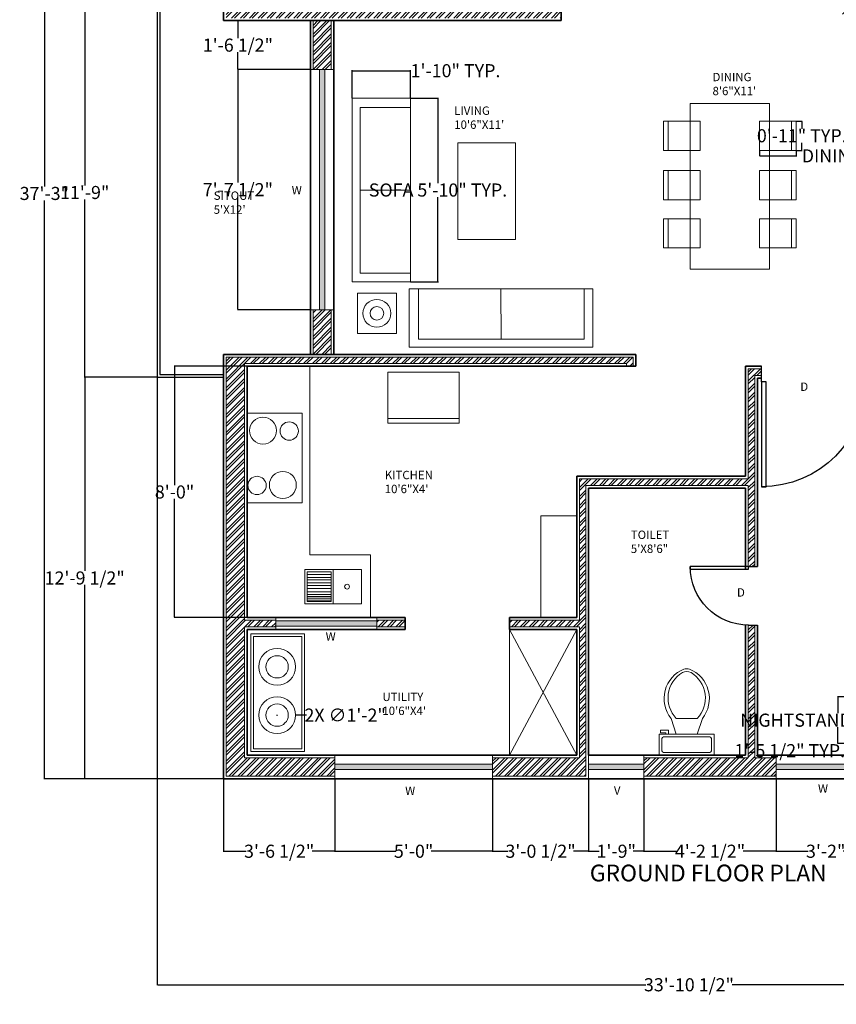
# Model space of a CAD drawing. Units: inches. Extents: x -340 to 394, y 381 to 1380.
# Tile 1 of 3: x -117 to 195, y 381 to 757. Entities that reach past the tile are written whole.
import ezdxf

# ---------------------------------------------------------------- set-up
doc = ezdxf.new("R2010")
doc.units = ezdxf.units.IN
doc.header["$MEASUREMENT"] = 0
for name, color, linetype, lineweight in [('A-ANNO-DIMS', 150, 'Continuous', 18), ('A-ANNO-TEXT', 11, 'Continuous', 18), ('A-AREA-IDEN', 11, 'Continuous', 18), ('A-EQPM', 130, 'Continuous', 18), ('A-FLOR', 150, 'Continuous', 25), ('A-FLOR-CASE', 130, 'Continuous', 20), ('A-FLOR-FIXT', 130, 'Continuous', 18), ('A-GLAZ-PATT', 220, 'Continuous', 13), ('A-WALL-FNSH', 150, 'Continuous', 18), ('A-WALL-PATT', 10, 'Continuous', 13), ('door', 200, 'Continuous', 25), ('fur', 130, 'Continuous', 18), ('wall', 150, 'Continuous', 35), ('wind', 220, 'Continuous', 20)]:
    doc.layers.add(name, color=color, linetype=linetype, lineweight=lineweight)
doc.styles.get("Standard").update_dxf_attribs({"font": 'arial.ttf'})
doc.dimstyles.get("Standard").update_dxf_attribs({"dimtxt": 5, "dimasz": 0.18, "dimexe": 0.18, "dimexo": 0.0625, "dimgap": 0.09, "dimtad": 0, "dimtih": 1, "dimtoh": 1, "dimdec": 0, "dimzin": 0, "dimdsep": 46, "dimlunit": 4, "dimtxsty": 'Standard', "dimcen": 0.09, "dimadec": 0, "dimazin": 0, "dimtfac": 1, "dimtdec": 0, "dimtofl": 0, "dimtmove": 0, "dimatfit": 3, "dimfxl": 1, "dimtolj": 1, "dimtzin": 0, "dimarcsym": 0})

# ---------------------------------------------------------------- blocks, each defined once
blk = doc.blocks.new('*U2')
for p, q in [((0, 0), (0, -6)), ((40, 0), (40, -6))]:
    blk.add_line(p, q)
blk.add_lwpolyline([(0, 0), (0, 40), (1.75, 40), (1.75, 0)], close=True)
blk.add_arc((0, 0), 40, 0, 90)
blk = doc.blocks.new('*U4')
for p, q in [((9.5, -6), (9.5, -2)), ((-10, -8.5), (-8, -8.5)), ((-10, -9.5), (-10, -8.5)), ((-7, -9.5), (-10, -9.5)), ((-8, -8.5), (-8, -8)), ((-7, -8), (-7, -9.5)), ((-4, -8), (-6, -14)), ((4, -8), (6, -14)), ((4, -14), (-4, -14))]:
    blk.add_line(p, q)
blk.add_lwpolyline([(10.5, -8), (10.5, 0), (-10.5, 0), (-10.5, -8)], close=True)
for points in [[(-9.5, -2), (-9.5, -6)], [(8.5, -1), (-8.5, -1)], [(-8.5, -7), (8.5, -7)]]:
    blk.add_lwpolyline(points)
for centre, radius, start, end in [((-8.62, -1.88), 0.884, 81.8699, 188.1301), ((8.62, -1.88), 0.884, 351.8699, 98.1301), ((-8.62, -6.12), 0.884, 171.8699, 278.1301), ((8.62, -6.12), 0.884, 261.8699, 8.1301), ((3.52, -21.58), 12.17, 141.4691, 247.9714), ((4.2, -21.82), 11.33, 136.3677, 238.9468), ((-3.52, -21.58), 12.17, 292.0284, 38.5307), ((-4.2, -21.82), 11.33, 301.053, 43.6321), ((0, -27.88), 4, 245.7318, 294.2682), ((0, -29), 4, 254.8605, 285.1395)]:
    blk.add_arc(centre, radius, start, end)
blk = doc.blocks.new('*D6')
at = {"layer": 'A-ANNO-DIMS', "color": 0, "lineweight": -2, "transparency": 16777216}
for p, q in [((-39.68, 914.2), (-108.24, 914.2)), ((-108.06, 914.02), (-108.06, 693.34)), ((-108.06, 467.38), (-108.06, 688.05)), ((-39.68, 467.2), (-108.24, 467.2))]:
    blk.add_line(p, q, dxfattribs=at)
at = {"layer": 'A-ANNO-DIMS', "color": 0, "transparency": 16777216}
for points in [[(-108.09, 914.02), (-108.03, 914.02), (-108.06, 914.2)], [(-108.09, 467.38), (-108.03, 467.38), (-108.06, 467.2)]]:
    blk.add_solid(points, dxfattribs=at)
at = {"layer": 'Defpoints', "color": 0, "transparency": 16777216}
for p in [(-39.62, 914.2), (-108.06, 467.2), (-39.62, 467.2)]:
    blk.add_point(p, dxfattribs=at)
at = {"layer": 'A-ANNO-DIMS', "color": 0, "transparency": 16777216, "insert": (-108.06, 690.7), "char_height": 5, "attachment_point": 5}
blk.add_mtext('\\A1;37\'-3"', dxfattribs=at)
blk = doc.blocks.new('SOFA-LIVING')
for p, q in [((3.51, 22.24), (3.51, 3.07)), ((35.05, 22.24), (35.15, 3.07)), ((66.79, 3.07), (66.79, 22.24)), ((3.51, 3.07), (66.79, 3.07))]:
    blk.add_line(p, q)
blk.add_lwpolyline([(70.1, 0), (0, 0), (0, 22.24), (70.1, 22.24)], close=True)
blk = doc.blocks.new('CHAIR-DINING')
blk.add_line((12.18, 11.15), (12.18, 0))
blk.add_lwpolyline([(0, 11.15), (14.01, 11.15), (14.01, 0), (0, 0)], close=True)
blk = doc.blocks.new('*D13')
at = {"layer": 'A-ANNO-DIMS', "color": 0, "lineweight": -2, "transparency": 16777216}
for p, q in [((197.74, 498.52), (194.94, 498.52)), ((195.12, 498.34), (195.12, 492.23)), ((195.12, 480.77), (195.12, 486.88)), ((197.74, 480.59), (194.94, 480.59))]:
    blk.add_line(p, q, dxfattribs=at)
at = {"layer": 'A-ANNO-DIMS', "color": 0, "transparency": 16777216}
for points in [[(195.09, 498.34), (195.15, 498.34), (195.12, 498.52)], [(195.09, 480.77), (195.15, 480.77), (195.12, 480.59)]]:
    blk.add_solid(points, dxfattribs=at)
at = {"layer": 'Defpoints', "color": 0, "transparency": 16777216}
for p in [(195.12, 498.52), (197.81, 498.52), (197.81, 480.59)]:
    blk.add_point(p, dxfattribs=at)
at = {"layer": 'A-ANNO-DIMS', "color": 0, "transparency": 16777216, "insert": (195.12, 489.55), "char_height": 5, "attachment_point": 5}
blk.add_mtext('\\A1;NIGHTSTAND 1\'-6" TYP.', dxfattribs=at)
blk = doc.blocks.new('*D14')
at = {"layer": 'A-ANNO-DIMS', "color": 0, "lineweight": -2, "transparency": 16777216}
for p, q in [((197.81, 477.9), (197.63, 477.9)), ((197.81, 480.52), (197.81, 477.72)), ((215.12, 477.9), (197.99, 477.9)), ((215.3, 480.52), (215.3, 477.72))]:
    blk.add_line(p, q, dxfattribs=at)
at = {"layer": 'A-ANNO-DIMS', "color": 0, "transparency": 16777216}
for points in [[(197.99, 477.93), (197.99, 477.87), (197.81, 477.9)], [(215.12, 477.93), (215.12, 477.87), (215.3, 477.9)]]:
    blk.add_solid(points, dxfattribs=at)
at = {"layer": 'Defpoints', "color": 0, "transparency": 16777216}
for p in [(197.81, 480.59), (197.81, 477.9), (215.3, 480.59)]:
    blk.add_point(p, dxfattribs=at)
at = {"layer": 'A-ANNO-DIMS', "color": 0, "transparency": 16777216, "insert": (176.71, 477.9), "char_height": 5, "attachment_point": 5}
blk.add_mtext('\\A1;1\'-5 1/2" TYP.', dxfattribs=at)
blk = doc.blocks.new('*D19')
at = {"layer": 'A-ANNO-DIMS', "color": 0, "lineweight": -2, "transparency": 16777216}
for p, q in [((31.88, 727.06), (42.51, 727.06)), ((42.33, 726.88), (42.33, 694.69)), ((42.33, 657.14), (42.33, 689.34)), ((31.88, 656.96), (42.51, 656.96))]:
    blk.add_line(p, q, dxfattribs=at)
at = {"layer": 'A-ANNO-DIMS', "color": 0, "transparency": 16777216}
for points in [[(42.3, 726.88), (42.36, 726.88), (42.33, 727.06)], [(42.3, 657.14), (42.36, 657.14), (42.33, 656.96)]]:
    blk.add_solid(points, dxfattribs=at)
at = {"layer": 'Defpoints', "color": 0, "transparency": 16777216}
for p in [(31.81, 727.06), (31.81, 656.96), (42.33, 656.96)]:
    blk.add_point(p, dxfattribs=at)
at = {"layer": 'A-ANNO-DIMS', "color": 0, "transparency": 16777216, "insert": (42.33, 692.01), "char_height": 5, "attachment_point": 5}
blk.add_mtext('\\A1;SOFA 5\'-10" TYP.', dxfattribs=at)
blk = doc.blocks.new('*D20')
at = {"layer": 'A-ANNO-DIMS', "color": 0, "lineweight": -2, "transparency": 16777216}
for p, q in [((9.57, 727.13), (9.57, 737.76)), ((9.75, 737.58), (31.63, 737.58)), ((31.81, 727.13), (31.81, 737.76)), ((31.81, 737.58), (31.99, 737.58))]:
    blk.add_line(p, q, dxfattribs=at)
at = {"layer": 'A-ANNO-DIMS', "color": 0, "transparency": 16777216}
for points in [[(9.75, 737.61), (9.75, 737.55), (9.57, 737.58)], [(31.63, 737.61), (31.63, 737.55), (31.81, 737.58)]]:
    blk.add_solid(points, dxfattribs=at)
at = {"layer": 'Defpoints', "color": 0, "transparency": 16777216}
for p in [(31.81, 737.58), (9.57, 727.06), (31.81, 727.06)]:
    blk.add_point(p, dxfattribs=at)
at = {"layer": 'A-ANNO-DIMS', "color": 0, "transparency": 16777216, "insert": (49.03, 737.58), "char_height": 5, "attachment_point": 5}
blk.add_mtext('\\A1;1\'-10" TYP.', dxfattribs=at)
blk = doc.blocks.new('*D23')
at = {"layer": 'A-ANNO-DIMS', "color": 0, "lineweight": -2, "transparency": 16777216}
for p, q in [((165.2, 707.1), (165.2, 704.88)), ((179.21, 707.1), (179.21, 704.88)), ((165.38, 705.06), (179.03, 705.06)), ((179.21, 705.06), (179.39, 705.06))]:
    blk.add_line(p, q, dxfattribs=at)
at = {"layer": 'A-ANNO-DIMS', "color": 0, "transparency": 16777216}
for points in [[(165.38, 705.09), (165.38, 705.03), (165.2, 705.06)], [(179.03, 705.09), (179.03, 705.03), (179.21, 705.06)]]:
    blk.add_solid(points, dxfattribs=at)
at = {"layer": 'Defpoints', "color": 0, "transparency": 16777216}
for p in [(165.2, 707.16), (179.21, 707.16), (179.21, 705.06)]:
    blk.add_point(p, dxfattribs=at)
at = {"layer": 'A-ANNO-DIMS', "color": 0, "transparency": 16777216, "insert": (219.63, 705.06), "char_height": 5, "attachment_point": 5}
blk.add_mtext('\\A1;DINING CHAIR 1\'-2" TYP.', dxfattribs=at)
blk = doc.blocks.new('*D24')
at = {"layer": 'A-ANNO-DIMS', "color": 0, "lineweight": -2, "transparency": 16777216}
for p, q in [((179.28, 718.31), (181.5, 718.31)), ((181.32, 718.13), (181.32, 715.38)), ((179.28, 707.16), (181.5, 707.16)), ((181.32, 707.34), (181.32, 710.09))]:
    blk.add_line(p, q, dxfattribs=at)
at = {"layer": 'A-ANNO-DIMS', "color": 0, "transparency": 16777216}
for points in [[(181.29, 718.13), (181.35, 718.13), (181.32, 718.31)], [(181.29, 707.34), (181.35, 707.34), (181.32, 707.16)]]:
    blk.add_solid(points, dxfattribs=at)
at = {"layer": 'Defpoints', "color": 0, "transparency": 16777216}
for p in [(179.21, 718.31), (181.32, 718.31), (179.21, 707.16)]:
    blk.add_point(p, dxfattribs=at)
at = {"layer": 'A-ANNO-DIMS', "color": 0, "transparency": 16777216, "insert": (181.32, 712.74), "char_height": 5, "attachment_point": 5}
blk.add_mtext('\\A1;0\'-11" TYP.', dxfattribs=at)
blk = doc.blocks.new('*D41')
at = {"layer": 'A-ANNO-DIMS', "color": 0, "lineweight": -2, "transparency": 16777216}
for p, q in [((-65, 620.5), (-92.82, 620.5)), ((-92.64, 620.32), (-92.64, 546.53)), ((-92.64, 467.38), (-92.64, 541.18)), ((-39.68, 467.2), (-92.82, 467.2))]:
    blk.add_line(p, q, dxfattribs=at)
at = {"layer": 'A-ANNO-DIMS', "color": 0, "transparency": 16777216}
for points in [[(-92.67, 620.32), (-92.61, 620.32), (-92.64, 620.5)], [(-92.67, 467.38), (-92.61, 467.38), (-92.64, 467.2)]]:
    blk.add_solid(points, dxfattribs=at)
at = {"layer": 'Defpoints', "color": 0, "transparency": 16777216}
for p in [(-92.64, 620.5), (-64.94, 620.5), (-39.62, 467.2)]:
    blk.add_point(p, dxfattribs=at)
at = {"layer": 'A-ANNO-DIMS', "color": 0, "transparency": 16777216, "insert": (-92.64, 543.85), "char_height": 5, "attachment_point": 5}
blk.add_mtext('\\A1;12\'-9 1/2"', dxfattribs=at)
blk = doc.blocks.new('*D42')
at = {"layer": 'A-ANNO-DIMS', "color": 0, "lineweight": -2, "transparency": 16777216}
for p, q in [((-65, 761.64), (-92.82, 761.64)), ((-92.64, 761.46), (-92.64, 693.71)), ((-92.64, 620.68), (-92.64, 688.43)), ((-65, 620.5), (-92.82, 620.5))]:
    blk.add_line(p, q, dxfattribs=at)
at = {"layer": 'A-ANNO-DIMS', "color": 0, "transparency": 16777216}
for points in [[(-92.67, 761.46), (-92.61, 761.46), (-92.64, 761.64)], [(-92.67, 620.68), (-92.61, 620.68), (-92.64, 620.5)]]:
    blk.add_solid(points, dxfattribs=at)
at = {"layer": 'Defpoints', "color": 0, "transparency": 16777216}
for p in [(-92.64, 761.64), (-64.94, 761.64), (-64.94, 620.5)]:
    blk.add_point(p, dxfattribs=at)
at = {"layer": 'A-ANNO-DIMS', "color": 0, "transparency": 16777216, "insert": (-92.64, 691.07), "char_height": 5, "attachment_point": 5}
blk.add_mtext('\\A1;11\'-9"', dxfattribs=at)
blk = doc.blocks.new('*D46')
at = {"layer": 'A-ANNO-DIMS', "color": 0, "lineweight": -2, "transparency": 16777216}
for p, q in [((-6.48, 737.98), (-34.3, 737.98)), ((-34.12, 737.8), (-34.12, 694.82)), ((-34.12, 646.49), (-34.12, 689.47)), ((-6.48, 646.31), (-34.3, 646.31))]:
    blk.add_line(p, q, dxfattribs=at)
at = {"layer": 'A-ANNO-DIMS', "color": 0, "transparency": 16777216}
for points in [[(-34.15, 737.8), (-34.09, 737.8), (-34.12, 737.98)], [(-34.15, 646.49), (-34.09, 646.49), (-34.12, 646.31)]]:
    blk.add_solid(points, dxfattribs=at)
at = {"layer": 'Defpoints', "color": 0, "transparency": 16777216}
for p in [(-34.12, 737.98), (-6.42, 737.98), (-6.42, 646.31)]:
    blk.add_point(p, dxfattribs=at)
at = {"layer": 'A-ANNO-DIMS', "color": 0, "transparency": 16777216, "insert": (-34.12, 692.15), "char_height": 5, "attachment_point": 5}
blk.add_mtext('\\A1;7\'-7 1/2"', dxfattribs=at)
blk = doc.blocks.new('*D47')
at = {"layer": 'A-ANNO-DIMS', "color": 0, "lineweight": -2, "transparency": 16777216}
for p, q in [((-6.48, 756.7), (-34.3, 756.7)), ((-34.12, 756.52), (-34.12, 750.02)), ((-34.12, 738.16), (-34.12, 744.67)), ((-6.48, 737.98), (-34.3, 737.98))]:
    blk.add_line(p, q, dxfattribs=at)
at = {"layer": 'A-ANNO-DIMS', "color": 0, "transparency": 16777216}
for points in [[(-34.15, 756.52), (-34.09, 756.52), (-34.12, 756.7)], [(-34.15, 738.16), (-34.09, 738.16), (-34.12, 737.98)]]:
    blk.add_solid(points, dxfattribs=at)
at = {"layer": 'Defpoints', "color": 0, "transparency": 16777216}
for p in [(-34.12, 756.7), (-6.42, 756.7), (-6.42, 737.98)]:
    blk.add_point(p, dxfattribs=at)
at = {"layer": 'A-ANNO-DIMS', "color": 0, "transparency": 16777216, "insert": (-34.12, 747.34), "char_height": 5, "attachment_point": 5}
blk.add_mtext('\\A1;1\'-6 1/2"', dxfattribs=at)
blk = doc.blocks.new('*D48')
at = {"layer": 'A-ANNO-DIMS', "color": 0, "lineweight": -2, "transparency": 16777216}
for p, q in [((-30.68, 624.7), (-58.5, 624.7)), ((-58.32, 624.52), (-58.32, 579.34)), ((-58.32, 528.88), (-58.32, 574.06)), ((-30.68, 528.7), (-58.5, 528.7))]:
    blk.add_line(p, q, dxfattribs=at)
at = {"layer": 'A-ANNO-DIMS', "color": 0, "transparency": 16777216}
for points in [[(-58.35, 624.52), (-58.29, 624.52), (-58.32, 624.7)], [(-58.35, 528.88), (-58.29, 528.88), (-58.32, 528.7)]]:
    blk.add_solid(points, dxfattribs=at)
at = {"layer": 'Defpoints', "color": 0, "transparency": 16777216}
for p in [(-58.32, 624.7), (-30.62, 624.7), (-30.62, 528.7)]:
    blk.add_point(p, dxfattribs=at)
at = {"layer": 'A-ANNO-DIMS', "color": 0, "transparency": 16777216, "insert": (-58.32, 576.7), "char_height": 5, "attachment_point": 5}
blk.add_mtext('\\A1;8\'-0"', dxfattribs=at)
blk = doc.blocks.new('*D49')
at = {"layer": 'A-ANNO-DIMS', "color": 0, "lineweight": -2, "transparency": 16777216}
for p, q in [((-39.62, 467.14), (-39.62, 439.32)), ((2.91, 467.14), (2.91, 439.32)), ((-39.44, 439.5), (-30.91, 439.5)), ((2.73, 439.5), (-5.8, 439.5))]:
    blk.add_line(p, q, dxfattribs=at)
at = {"layer": 'A-ANNO-DIMS', "color": 0, "transparency": 16777216}
for points in [[(-39.44, 439.53), (-39.44, 439.47), (-39.62, 439.5)], [(2.73, 439.53), (2.73, 439.47), (2.91, 439.5)]]:
    blk.add_solid(points, dxfattribs=at)
at = {"layer": 'Defpoints', "color": 0, "transparency": 16777216}
for p in [(-39.62, 467.2), (2.91, 467.2), (-39.62, 439.5)]:
    blk.add_point(p, dxfattribs=at)
at = {"layer": 'A-ANNO-DIMS', "color": 0, "transparency": 16777216, "insert": (-18.35, 439.5), "char_height": 5, "attachment_point": 5}
blk.add_mtext('\\A1;3\'-6 1/2"', dxfattribs=at)
blk = doc.blocks.new('*D50')
at = {"layer": 'A-ANNO-DIMS', "color": 0, "lineweight": -2, "transparency": 16777216}
for p, q in [((2.91, 467.14), (2.91, 439.32)), ((63.15, 467.14), (63.15, 439.32)), ((3.09, 439.5), (26.29, 439.5)), ((62.97, 439.5), (39.76, 439.5))]:
    blk.add_line(p, q, dxfattribs=at)
at = {"layer": 'A-ANNO-DIMS', "color": 0, "transparency": 16777216}
for points in [[(3.09, 439.53), (3.09, 439.47), (2.91, 439.5)], [(62.97, 439.53), (62.97, 439.47), (63.15, 439.5)]]:
    blk.add_solid(points, dxfattribs=at)
at = {"layer": 'Defpoints', "color": 0, "transparency": 16777216}
for p in [(2.91, 467.2), (63.15, 467.2), (2.91, 439.5)]:
    blk.add_point(p, dxfattribs=at)
at = {"layer": 'A-ANNO-DIMS', "color": 0, "transparency": 16777216, "insert": (33.03, 439.5), "char_height": 5, "attachment_point": 5}
blk.add_mtext('\\A1;5\'-0"', dxfattribs=at)
blk = doc.blocks.new('*D51')
at = {"layer": 'A-ANNO-DIMS', "color": 0, "lineweight": -2, "transparency": 16777216}
for p, q in [((63.15, 467.14), (63.15, 439.32)), ((99.88, 467.14), (99.88, 439.32)), ((63.33, 439.5), (68.96, 439.5)), ((99.7, 439.5), (94.07, 439.5))]:
    blk.add_line(p, q, dxfattribs=at)
at = {"layer": 'A-ANNO-DIMS', "color": 0, "transparency": 16777216}
for points in [[(63.33, 439.53), (63.33, 439.47), (63.15, 439.5)], [(99.7, 439.53), (99.7, 439.47), (99.88, 439.5)]]:
    blk.add_solid(points, dxfattribs=at)
at = {"layer": 'Defpoints', "color": 0, "transparency": 16777216}
for p in [(63.15, 467.2), (99.88, 467.2), (63.15, 439.5)]:
    blk.add_point(p, dxfattribs=at)
at = {"layer": 'A-ANNO-DIMS', "color": 0, "transparency": 16777216, "insert": (81.52, 439.5), "char_height": 5, "attachment_point": 5}
blk.add_mtext('\\A1;3\'-0 1/2"', dxfattribs=at)
blk = doc.blocks.new('*D52')
at = {"layer": 'A-ANNO-DIMS', "color": 0, "lineweight": -2, "transparency": 16777216}
for p, q in [((99.88, 467.14), (99.88, 439.32)), ((121.02, 467.14), (121.02, 439.32)), ((100.06, 439.5), (103.95, 439.5)), ((120.84, 439.5), (116.95, 439.5))]:
    blk.add_line(p, q, dxfattribs=at)
at = {"layer": 'A-ANNO-DIMS', "color": 0, "transparency": 16777216}
for points in [[(100.06, 439.53), (100.06, 439.47), (99.88, 439.5)], [(120.84, 439.53), (120.84, 439.47), (121.02, 439.5)]]:
    blk.add_solid(points, dxfattribs=at)
at = {"layer": 'Defpoints', "color": 0, "transparency": 16777216}
for p in [(99.88, 467.2), (121.02, 467.2), (99.88, 439.5)]:
    blk.add_point(p, dxfattribs=at)
at = {"layer": 'A-ANNO-DIMS', "color": 0, "transparency": 16777216, "insert": (110.45, 439.5), "char_height": 5, "attachment_point": 5}
blk.add_mtext('\\A1;1\'-9"', dxfattribs=at)
blk = doc.blocks.new('*D53')
at = {"layer": 'A-ANNO-DIMS', "color": 0, "lineweight": -2, "transparency": 16777216}
for p, q in [((121.02, 467.14), (121.02, 439.32)), ((171.54, 467.14), (171.54, 439.32)), ((121.2, 439.5), (133.62, 439.5)), ((171.36, 439.5), (158.94, 439.5))]:
    blk.add_line(p, q, dxfattribs=at)
at = {"layer": 'A-ANNO-DIMS', "color": 0, "transparency": 16777216}
for points in [[(121.2, 439.53), (121.2, 439.47), (121.02, 439.5)], [(171.36, 439.53), (171.36, 439.47), (171.54, 439.5)]]:
    blk.add_solid(points, dxfattribs=at)
at = {"layer": 'Defpoints', "color": 0, "transparency": 16777216}
for p in [(121.02, 467.2), (171.54, 467.2), (121.02, 439.5)]:
    blk.add_point(p, dxfattribs=at)
at = {"layer": 'A-ANNO-DIMS', "color": 0, "transparency": 16777216, "insert": (146.28, 439.5), "char_height": 5, "attachment_point": 5}
blk.add_mtext('\\A1;4\'-2 1/2"', dxfattribs=at)
blk = doc.blocks.new('*D54')
at = {"layer": 'A-ANNO-DIMS', "color": 0, "lineweight": -2, "transparency": 16777216}
for p, q in [((171.54, 467.14), (171.54, 439.32)), ((209.39, 467.14), (209.39, 439.32)), ((171.72, 439.5), (183.73, 439.5)), ((209.21, 439.5), (197.2, 439.5))]:
    blk.add_line(p, q, dxfattribs=at)
at = {"layer": 'A-ANNO-DIMS', "color": 0, "transparency": 16777216}
for points in [[(171.72, 439.53), (171.72, 439.47), (171.54, 439.5)], [(209.21, 439.53), (209.21, 439.47), (209.39, 439.5)]]:
    blk.add_solid(points, dxfattribs=at)
at = {"layer": 'Defpoints', "color": 0, "transparency": 16777216}
for p in [(171.54, 467.2), (209.39, 467.2), (171.54, 439.5)]:
    blk.add_point(p, dxfattribs=at)
at = {"layer": 'A-ANNO-DIMS', "color": 0, "transparency": 16777216, "insert": (190.47, 439.5), "char_height": 5, "attachment_point": 5}
blk.add_mtext('\\A1;3\'-2"', dxfattribs=at)
blk = doc.blocks.new('*D58')
at = {"layer": 'A-ANNO-DIMS', "color": 0, "lineweight": -2, "transparency": 16777216}
for p, q in [((-64.94, 620.44), (-64.94, 388.32)), ((341.38, 467.14), (341.38, 388.32)), ((-64.76, 388.5), (121.78, 388.5)), ((341.2, 388.5), (154.67, 388.5))]:
    blk.add_line(p, q, dxfattribs=at)
at = {"layer": 'A-ANNO-DIMS', "color": 0, "transparency": 16777216}
for points in [[(-64.76, 388.53), (-64.76, 388.47), (-64.94, 388.5)], [(341.2, 388.53), (341.2, 388.47), (341.38, 388.5)]]:
    blk.add_solid(points, dxfattribs=at)
at = {"layer": 'Defpoints', "color": 0, "transparency": 16777216}
for p in [(-64.94, 620.5), (341.38, 467.2), (341.38, 388.5)]:
    blk.add_point(p, dxfattribs=at)
at = {"layer": 'A-ANNO-DIMS', "color": 0, "transparency": 16777216, "insert": (138.22, 388.5), "char_height": 5, "attachment_point": 5}
blk.add_mtext('\\A1;33\'-10 1/2"', dxfattribs=at)
blk = doc.blocks.new('*D59')
at = {"layer": 'A-ANNO-DIMS', "color": 0, "lineweight": -2, "transparency": 16777216}
for p, q in [((-19.22, 491.48), (-19.04, 491.48)), ((-19.13, 491.39), (-19.13, 491.57)), ((-7.87, 491.48), (-11.91, 491.48))]:
    blk.add_line(p, q, dxfattribs=at)
at = {"layer": 'A-ANNO-DIMS', "color": 0, "transparency": 16777216}
blk.add_solid([(-11.91, 491.51), (-11.91, 491.45), (-12.09, 491.48)], dxfattribs=at)
at = {"layer": 'Defpoints', "color": 0, "transparency": 16777216}
for p in [(-26.16, 491.48), (-12.09, 491.48)]:
    blk.add_point(p, dxfattribs=at)
at = {"layer": 'A-ANNO-DIMS', "color": 0, "transparency": 16777216, "insert": (6.87, 491.48), "char_height": 5, "attachment_point": 5}
blk.add_mtext('\\A1;2X ∅1\'-2"', dxfattribs=at)

msp = doc.modelspace()

# ---------------------------------------------------------------- hatches: boundary and pattern name
at = {"layer": 'A-GLAZ-PATT'}
h = msp.add_hatch(color=256, dxfattribs=at)
h.dxf.hatch_style = 1
h.paths.add_polyline_path([(58.56, 910.7), (-1.68, 910.7), (-1.68, 908.7), (58.56, 908.7)])
h.paths.add_polyline_path([(115.02, 910.7), (93.88, 910.7), (93.88, 908.7), (115.02, 908.7)])
h.paths.add_polyline_path([(206.8, 910.7), (185.67, 910.7), (185.67, 908.7), (206.8, 908.7)])
h.paths.add_polyline_path([(308.48, 910.7), (236.12, 910.7), (236.12, 908.7), (308.48, 908.7)])
h.paths.add_polyline_path([(337.88, 852.47), (335.88, 852.47), (335.88, 801.11), (337.88, 801.11)])
h.paths.add_polyline_path([(-34.12, 843.05), (-36.12, 843.05), (-36.12, 791.69), (-34.12, 791.69)])
h.paths.add_polyline_path([(-0.92, 737.98), (-2.92, 737.98), (-2.92, 646.31), (-0.92, 646.31)])
h.paths.add_polyline_path([(337.88, 685.13), (335.88, 685.13), (335.88, 633.76), (337.88, 633.76)])
h.paths.add_polyline_path([(19, 527.45), (-19.67, 527.45), (-19.67, 525.45), (19, 525.45)])
h.paths.add_polyline_path([(63.15, 472.7), (2.91, 472.7), (2.91, 470.7), (63.15, 470.7)])
h.paths.add_polyline_path([(121.02, 472.7), (99.88, 472.7), (99.88, 470.7), (121.02, 470.7)])
h.paths.add_polyline_path([(310.81, 472.7), (272.96, 472.7), (272.96, 470.7), (310.81, 470.7)])
h.paths.add_polyline_path([(209.39, 472.7), (171.54, 472.7), (171.54, 470.7), (209.39, 470.7)])
at = {"layer": 'A-WALL-PATT'}
h = msp.add_hatch(dxfattribs=at)
h.set_pattern_fill('ANSI32', color=256, scale=6.4)
h.paths.add_polyline_path([(211.38, 905.2), (208.88, 905.2), (208.88, 859.96), (211.38, 859.96)])
h.paths.add_polyline_path([(211.38, 833.2), (208.88, 833.2), (208.88, 808.2), (146.36, 808.2), (146.36, 805.7), (211.38, 805.7)])
h.paths.add_polyline_path([(92.88, 905.2), (90.38, 905.2), (90.38, 805.7), (119.27, 805.7), (119.27, 808.2), (92.88, 808.2)])
h.paths.add_polyline_path([(1.58, 756.7), (-5.42, 756.7), (-5.42, 737.98), (1.58, 737.98)], flags=17)
h.paths.add_polyline_path([(1.58, 646.31), (-5.42, 646.31), (-5.42, 629.2), (1.58, 629.2)])
h.paths.add_polyline_path([(340.38, 697.15), (335.38, 697.15, -0.012506), (333.38, 697.2), (333.38, 685.13), (340.38, 685.13)])
h.paths.add_polyline_path([(29.76, 527.7), (19, 527.7), (19, 525.2), (29.76, 525.2)], flags=17)
h.paths.add_polyline_path([(98.88, 579.2), (160.88, 579.2), (160.88, 548.2), (161.03, 548.2), (163.38, 548.2), (163.38, 621.2), (165.94, 621.2), (165.94, 623.7), (160.88, 623.7), (160.88, 581.7), (96.38, 581.7), (96.38, 527.7), (69.71, 527.7), (69.71, 525.2), (96.38, 525.2), (96.38, 475.2), (63.15, 475.2), (63.15, 468.2), (98.88, 468.2)])
h.paths.add_polyline_path([(171.54, 475.2), (163.38, 475.2), (163.38, 525.87), (160.88, 525.87), (160.88, 475.2), (121.02, 475.2), (121.02, 468.2), (159.88, 468.2), (171.54, 468.2)])
h.paths.add_polyline_path([(272.96, 475.2), (209.39, 475.2), (209.39, 468.2), (272.96, 468.2)], flags=17)
h.paths.add_polyline_path([(340.38, 620.2), (340.38, 633.76), (333.38, 633.76), (333.38, 623.7), (205.94, 623.7), (205.94, 621.2), (333.38, 621.2), (333.38, 475.2), (310.81, 475.2), (310.81, 468.2), (340.38, 468.2)])
h = msp.add_hatch(dxfattribs=at)
h.set_pattern_fill('ANSI32', color=256, scale=6.4)
h.paths.add_polyline_path([(116.88, 628.2), (-38.62, 628.2), (-38.62, 528.7), (-38.62, 468.2), (2.91, 468.2), (2.91, 475.2), (-31.62, 475.2), (-31.62, 525.2), (-19.67, 525.2), (-19.67, 527.7), (-31.62, 527.7), (-31.62, 625.7), (114.38, 625.7), (114.38, 624.7), (116.88, 624.7)])
h.paths.add_polyline_path([(-31.62, 791.69), (-38.62, 791.69), (-38.62, 757.7), (89.38, 757.7), (89.38, 760.2), (-31.62, 760.2)])
h.paths.add_polyline_path([(340.38, 801.11), (333.38, 801.11), (333.38, 760.2), (332.38, 760.2), (196.87, 760.2), (196.87, 757.7), (332.38, 757.7), (333.38, 757.7), (333.38, 746.4), (333.38, 737.15), (335.38, 737.15), (340.38, 737.15), (340.38, 756.7)])

# ---------------------------------------------------------------- linework, layer by layer
at = {"layer": 'A-EQPM'}
msp.add_line((23.15, 604.76), (50.43, 604.76), dxfattribs=at)
for points in [[(23.15, 622.5), (50.43, 622.5), (50.43, 602.95), (23.15, 602.95)], [(-9.61, 606.76), (-30.62, 606.76), (-30.62, 572.51), (-9.61, 572.51)], [(-29.16, 477.57), (-8.71, 477.57), (-8.71, 522.51), (-29.16, 522.51)], [(-28.16, 478.57), (-9.71, 478.57), (-9.71, 521.51), (-28.16, 521.51)]]:
    msp.add_lwpolyline(points, close=True, dxfattribs=at)
for centre, radius in [((-24.54, 600.14), 5.15), ((-14.51, 599.96), 3.49), ((-16.95, 579.37), 5.15), ((-26.79, 579.19), 3.49), ((-19.13, 509.93), 7.04), ((-19.13, 509.93), 4.25), ((-19.13, 491.48), 7.04), ((-19.13, 491.48), 4.25)]:
    msp.add_circle(centre, radius, dxfattribs=at)
at = {"layer": 'A-FLOR'}
for p, q in [((-64.94, 761.64), (-64.94, 620.5)), ((-63.94, 760.64), (-63.94, 621.5)), ((-64.94, 620.5), (-39.62, 620.5)), ((-63.94, 621.5), (-39.62, 621.5))]:
    msp.add_line(p, q, dxfattribs=at)
at = {"layer": 'A-FLOR-CASE'}
for p, q in [((-30.62, 624.7), (-6.62, 624.7)), ((-6.62, 624.7), (-6.62, 552.7)), ((16.58, 552.7), (-6.62, 552.7)), ((16.58, 528.7), (16.58, 552.7)), ((69.71, 524.2), (69.71, 476.2)), ((69.71, 476.2), (95.38, 524.2)), ((69.71, 524.2), (95.38, 476.2))]:
    msp.add_line(p, q, dxfattribs=at)
msp.add_lwpolyline([(95.38, 528.7), (81.6, 528.7), (81.6, 567.62), (95.38, 567.62)], close=True, dxfattribs=at)
at = {"layer": 'A-FLOR-FIXT'}
for p, q in [((2.31, 534.03), (2.31, 547.03)), ((-7.69, 545.2), (1.48, 545.2)), ((-7.62, 544.09), (1.55, 544.09)), ((-7.62, 543.12), (1.55, 543.12)), ((-7.62, 542.05), (1.55, 542.05)), ((-7.62, 540.97), (1.55, 540.97)), ((-7.62, 539.79), (1.55, 539.79)), ((-7.62, 538.57), (1.55, 538.57)), ((-7.62, 537.54), (1.55, 537.54)), ((-7.62, 536.79), (1.55, 536.79)), ((-7.62, 536.18), (1.55, 536.18)), ((-7.62, 535.35), (1.55, 535.35))]:
    msp.add_line(p, q, dxfattribs=at)
for points in [[(13.1, 547.03), (-8.48, 547.03), (-8.48, 534.03), (13.1, 534.03)], [(-7.69, 534.82), (1.48, 534.82), (1.48, 546.2), (-7.69, 546.2)]]:
    msp.add_lwpolyline(points, close=True, dxfattribs=at)
msp.add_circle((7.6, 540.53), 0.928, dxfattribs=at)
at = {"layer": 'A-WALL-FNSH'}
for p, q in [((-5.42, 737.98), (-5.42, 756.7)), ((1.58, 737.98), (1.58, 756.7)), ((-5.42, 629.2), (-5.42, 646.31)), ((1.58, 629.2), (1.58, 646.31)), ((-38.62, 528.7), (-38.62, 628.2)), ((-38.62, 628.2), (116.88, 628.2)), ((116.88, 628.2), (116.88, 624.7)), ((-31.62, 527.7), (-31.62, 625.7)), ((-31.62, 625.7), (114.38, 625.7)), ((114.38, 625.7), (114.38, 624.7)), ((160.88, 581.7), (160.88, 623.7)), ((160.88, 623.7), (165.94, 623.7)), ((163.38, 548.2), (163.38, 621.2)), ((163.38, 621.2), (165.94, 621.2)), ((96.38, 581.7), (160.88, 581.7)), ((96.38, 527.7), (96.38, 581.7)), ((98.88, 468.2), (98.88, 579.2)), ((98.88, 579.2), (160.88, 579.2)), ((160.88, 548.19), (160.88, 579.2)), ((159.88, 548.2), (160.88, 548.19)), ((-38.62, 468.2), (-38.62, 528.7)), ((-31.62, 527.7), (-19.67, 527.7)), ((29.76, 527.7), (19, 527.7)), ((96.38, 527.7), (69.71, 527.7)), ((-31.62, 475.2), (-31.62, 525.2)), ((-19.67, 525.2), (-31.62, 525.2)), ((29.76, 525.2), (19, 525.2)), ((96.38, 525.2), (69.71, 525.2)), ((96.38, 475.2), (96.38, 525.2)), ((160.88, 475.2), (160.88, 525.9)), ((163.38, 475.2), (163.38, 525.87)), ((2.91, 475.2), (-31.62, 475.2)), ((96.38, 475.2), (63.15, 475.2)), ((160.88, 475.2), (121.02, 475.2)), ((171.54, 475.2), (163.38, 475.2)), ((2.91, 468.2), (-38.62, 468.2)), ((98.88, 468.2), (63.15, 468.2)), ((159.88, 468.2), (121.02, 468.2)), ((171.54, 468.2), (159.88, 468.2))]:
    msp.add_line(p, q, dxfattribs=at)
at = {"layer": 'fur'}
for points in [[(168.94, 725.06), (138.74, 725.06), (138.74, 661.81), (168.94, 661.81)], [(49.95, 673.16), (71.97, 673.16), (71.97, 710.04), (49.95, 710.04)], [(26.42, 652.68), (11.52, 652.68), (11.52, 637.17), (26.42, 637.17)]]:
    msp.add_lwpolyline(points, close=True, dxfattribs=at)
for radius in [5.32, 2.61]:
    msp.add_circle((18.97, 644.92), radius, dxfattribs=at)
at = {"layer": 'wall'}
for p, q in [((-39.62, 756.7), (-39.62, 914.2)), ((-39.62, 791.69), (-39.62, 756.7)), ((89.38, 761.2), (89.38, 756.7)), ((-39.62, 756.7), (89.38, 756.7)), ((-39.62, 756.7), (89.38, 756.7)), ((-6.42, 629.2), (-6.42, 756.7)), ((-6.42, 737.98), (-6.42, 756.7)), ((2.58, 629.2), (2.58, 756.7)), ((2.58, 737.98), (2.58, 756.7)), ((-6.42, 629.2), (-6.42, 646.31)), ((2.58, 646.31), (2.58, 629.2)), ((-39.62, 528.7), (-39.62, 629.2)), ((-39.62, 629.2), (117.88, 629.2)), ((-39.62, 467.2), (-39.62, 629.2)), ((-39.62, 629.2), (-6.42, 629.2)), ((2.58, 629.2), (117.88, 629.2)), ((117.88, 629.2), (117.88, 624.7)), ((117.88, 629.2), (117.88, 624.7)), ((-30.62, 528.7), (-30.62, 624.7)), ((-30.62, 624.7), (113.38, 624.7)), ((113.38, 624.7), (-30.62, 624.7)), ((-30.62, 624.7), (-30.62, 528.7)), ((113.38, 624.7), (117.88, 624.7)), ((159.88, 624.7), (165.94, 624.7)), ((159.88, 582.7), (159.88, 624.7)), ((159.88, 582.7), (159.88, 624.7)), ((159.88, 624.7), (165.94, 624.7)), ((164.38, 620.2), (165.94, 620.2)), ((164.38, 548.2), (164.38, 620.2)), ((165.94, 620.2), (164.38, 620.2)), ((164.38, 620.2), (164.38, 548.2)), ((95.38, 582.7), (159.88, 582.7)), ((95.38, 528.7), (95.38, 582.7)), ((95.38, 528.7), (95.38, 582.7)), ((95.38, 582.7), (159.88, 582.7)), ((99.88, 476.2), (99.88, 578.2)), ((99.88, 578.2), (159.88, 578.2)), ((159.88, 578.2), (99.88, 578.2)), ((99.88, 578.2), (99.88, 476.2)), ((159.88, 547.22), (159.88, 578.2)), ((159.88, 548.2), (159.88, 578.2)), ((-39.62, 528.7), (-39.62, 536.7)), ((-39.62, 467.2), (-39.62, 528.7)), ((29.76, 528.7), (-30.62, 528.7)), ((-30.62, 528.7), (-19.67, 528.7)), ((29.76, 524.2), (29.76, 528.7)), ((95.38, 528.7), (69.71, 528.7)), ((69.71, 524.2), (69.71, 528.7)), ((69.71, 528.7), (95.38, 528.7)), ((-30.62, 476.2), (-30.62, 524.2)), ((29.76, 524.2), (-30.62, 524.2)), ((-19.67, 524.2), (-30.62, 524.2)), ((-30.62, 524.2), (-30.62, 476.2)), ((95.38, 524.2), (69.71, 524.2)), ((95.38, 524.2), (69.71, 524.2)), ((95.38, 476.2), (95.38, 524.2)), ((95.38, 476.2), (95.38, 524.2)), ((159.88, 476.2), (159.88, 525.9)), ((159.88, 525.9), (159.88, 476.2)), ((164.38, 476.2), (164.38, 525.87)), ((164.38, 476.2), (164.38, 525.87)), ((95.38, 476.2), (-30.62, 476.2)), ((-30.62, 476.2), (2.91, 476.2)), ((63.15, 476.2), (95.38, 476.2)), ((159.88, 476.2), (99.88, 476.2)), ((159.88, 476.2), (121.02, 476.2)), ((332.38, 476.2), (164.38, 476.2)), ((171.54, 476.2), (164.38, 476.2)), ((95.38, 467.2), (-39.62, 467.2)), ((2.91, 467.2), (-39.62, 467.2)), ((99.88, 467.2), (63.15, 467.2)), ((159.88, 467.2), (95.38, 467.2)), ((171.54, 467.2), (121.02, 467.2)), ((341.38, 467.2), (159.88, 467.2))]:
    msp.add_line(p, q, dxfattribs=at)
at = {"layer": 'wind'}
for p, q in [((-2.92, 646.31), (-2.92, 737.98)), ((-0.92, 646.31), (-0.92, 737.98)), ((-19.67, 527.45), (19, 527.45)), ((-19.67, 525.45), (19, 525.45)), ((2.91, 472.7), (63.15, 472.7)), ((2.91, 472.7), (63.15, 472.7)), ((2.91, 470.7), (63.15, 470.7)), ((99.88, 472.7), (121.02, 472.7)), ((99.88, 470.7), (121.02, 470.7)), ((171.54, 472.7), (209.39, 472.7)), ((171.54, 470.7), (209.39, 470.7))]:
    msp.add_line(p, q, dxfattribs=at)
for points in [[(2.58, 646.31), (-6.42, 646.31), (-6.42, 737.98), (2.58, 737.98)], [(-19.67, 528.7), (19, 528.7), (19, 524.2), (-19.67, 524.2)], [(2.91, 476.2), (63.15, 476.2), (63.15, 467.2), (2.91, 467.2)], [(99.88, 467.2), (121.02, 467.2), (121.02, 476.2), (99.88, 476.2)], [(171.54, 476.2), (209.39, 476.2), (209.39, 467.2), (171.54, 467.2)]]:
    msp.add_lwpolyline(points, close=True, dxfattribs=at)

# ---------------------------------------------------------------- block references
at = {"layer": 'A-FLOR-FIXT', "xscale": -1, "rotation": 180}
msp.add_blockref('*U4', (137.36, 476.2), dxfattribs=at)
at = {"layer": 'door', "xscale": -1, "rotation": 180}
msp.add_blockref('*U2', (165.94, 618.7), dxfattribs=at)
at = {"layer": 'door', "xscale": -0.5582468036305918, "yscale": 0.5582468036305918, "zscale": 0.5582468036305918, "rotation": 90}
msp.add_blockref('*U2', (161.03, 548.2), dxfattribs=at)
at = {"layer": 'fur', "rotation": 270.0000000000001}
msp.add_blockref('SOFA-LIVING', (9.57, 727.06), dxfattribs=at)
at = {"layer": 'fur', "extrusion": (0, 0, -1), "zscale": -1}
for p in [(-142.49, 707.16), (-142.49, 688.27), (-142.49, 669.92)]:
    msp.add_blockref('CHAIR-DINING', p, dxfattribs=at)
at = {"layer": 'fur'}
for name, p in [('CHAIR-DINING', (165.2, 707.16)), ('CHAIR-DINING', (165.2, 688.27)), ('CHAIR-DINING', (165.2, 669.92)), ('SOFA-LIVING', (31.34, 632))]:
    msp.add_blockref(name, p, dxfattribs=at)

# ---------------------------------------------------------------- texts
at = {"layer": 'A-ANNO-TEXT', "attachment_point": 1}
for s, width, gutter_width, insert, char_height in [('W', 932.3287, 16, (-13.54, 693.5), 3.2), ('D', 932.3287, 16, (180.76, 618.5), 3.2), ('D', 932.3287, 16, (156.58, 539.93), 3.2), ('W', 932.3287, 16, (-0.58, 523.1), 3.2), ('W', 932.3287, 16, (29.79, 464.2), 3.2), ('V', 932.3287, 16, (109.54, 464.31), 3.2), ('W', 932.3287, 16, (187.52, 465.03), 3.2), ('GROUND FLOOR PLAN', 1864.6573, 32, (100.33, 434.38), 6.4)]:
    msp.add_mtext_dynamic_manual_height_columns(s, width=width, gutter_width=gutter_width, heights=[0], dxfattribs=dict(at, insert=insert, char_height=char_height))
at = {"layer": 'A-AREA-IDEN', "char_height": 3.2, "attachment_point": 1}
for s, insert in [('DINING\\P8\'6"X11\'', (147.22, 736.76)), ('LIVING\\P10\'6"X11\'', (48.54, 723.91)), ("SITOUT\\P5'X12'", (-43.36, 691.46)), ('KITCHEN\\P10\'6"X4\'', (22, 584.78)), ('TOILET\\P5\'X8\'6"', (116.01, 561.95)), ('UTILITY\\P10\'6"X4\'', (21.09, 500.05))]:
    msp.add_mtext_dynamic_manual_height_columns(s, width=932.3287, gutter_width=16, heights=[0], dxfattribs=dict(at, insert=insert))

# ---------------------------------------------------------------- dimensions: what is measured, and where the dimension line sits
at = {"layer": 'A-ANNO-DIMS'}
for base, p1, p2, angle, override, picture, middle in [((-108.06, 467.2), (-39.62, 914.2), (-39.62, 467.2), 90, {"dimclrd": 0, "dimclre": 0, "dimclrt": 0}, '*D6', (-108.06, 690.7)), ((-92.64, 761.64), (-64.94, 620.5), (-64.94, 761.64), 90, {"dimdec": 1, "dimlfac": 1, "dimrnd": 0, "dimzin": 1, "dimdsep": 46, "dimlunit": 4, "dimfrac": 2}, '*D42', (-92.64, 691.07)), ((-34.12, 756.7), (-6.42, 737.98), (-6.42, 756.7), 90, {"dimdec": 1, "dimlfac": 1, "dimrnd": 0, "dimzin": 1, "dimdsep": 46, "dimlunit": 4, "dimfrac": 2}, '*D47', (-34.12, 747.34)), ((-34.12, 737.98), (-6.42, 646.31), (-6.42, 737.98), 90, {"dimdec": 1, "dimlfac": 1, "dimrnd": 0, "dimzin": 1, "dimdsep": 46, "dimlunit": 4, "dimfrac": 2}, '*D46', (-34.12, 692.15)), ((-58.32, 624.7), (-30.62, 528.7), (-30.62, 624.7), 90, {"dimdec": 1, "dimlfac": 1, "dimrnd": 0, "dimzin": 1, "dimdsep": 46, "dimlunit": 4, "dimfrac": 2}, '*D48', (-58.32, 576.7)), ((-92.64, 620.5), (-39.62, 467.2), (-64.94, 620.5), 90, {"dimdec": 1, "dimlfac": 1, "dimrnd": 0, "dimzin": 1, "dimdsep": 46, "dimlunit": 4, "dimfrac": 2}, '*D41', (-92.64, 543.85)), ((-39.62, 439.5), (2.91, 467.2), (-39.62, 467.2), 180, {"dimdec": 1, "dimlfac": 1, "dimrnd": 0, "dimzin": 1, "dimdsep": 46, "dimlunit": 4, "dimfrac": 2}, '*D49', (-18.35, 439.5)), ((2.91, 439.5), (63.15, 467.2), (2.91, 467.2), 180, {"dimdec": 1, "dimlfac": 1, "dimrnd": 0, "dimzin": 1, "dimdsep": 46, "dimlunit": 4, "dimfrac": 2}, '*D50', (33.03, 439.5)), ((63.15, 439.5), (99.88, 467.2), (63.15, 467.2), 180, {"dimdec": 1, "dimlfac": 1, "dimrnd": 0, "dimzin": 1, "dimdsep": 46, "dimlunit": 4, "dimfrac": 2}, '*D51', (81.52, 439.5)), ((99.88, 439.5), (121.02, 467.2), (99.88, 467.2), 180, {"dimdec": 1, "dimlfac": 1, "dimrnd": 0, "dimzin": 1, "dimdsep": 46, "dimlunit": 4, "dimfrac": 2}, '*D52', (110.45, 439.5)), ((121.02, 439.5), (171.54, 467.2), (121.02, 467.2), 180, {"dimdec": 1, "dimlfac": 1, "dimrnd": 0, "dimzin": 1, "dimdsep": 46, "dimlunit": 4, "dimfrac": 2}, '*D53', (146.28, 439.5)), ((171.5386, 439.4996), (209.3945, 467.1996), (171.5386, 467.1996), 180, {"dimdec": 1, "dimlfac": 1, "dimrnd": 0, "dimzin": 1, "dimdsep": 46, "dimlunit": 4, "dimfrac": 2}, '*D54', (190.4665, 439.4996))]:
    dim = msp.add_linear_dim(base=base, p1=p1, p2=p2, angle=angle, dimstyle='Standard', override=override, dxfattribs=at)
    dim.commit()
    dim.dimension.update_dxf_attribs({"geometry": picture, "text_midpoint": middle})
for base, p1, p2, text, picture, middle in [((31.81, 737.58), (9.57, 727.06), (31.81, 727.06), '<> TYP.', '*D20', (49.03, 737.58)), ((179.21, 705.06), (165.2, 707.16), (179.21, 707.16), 'DINING CHAIR <> TYP.', '*D23', (219.63, 705.06))]:
    dim = msp.add_linear_dim(base=base, p1=p1, p2=p2, text=text, dimstyle='Standard', override={"dimdec": 1, "dimlfac": 1, "dimrnd": 0, "dimzin": 1, "dimdsep": 46, "dimlunit": 4, "dimfrac": 2}, dxfattribs=at)
    dim.commit()
    dim.dimension.update_dxf_attribs({"geometry": picture, "text_midpoint": middle})
for base, p1, p2, angle, text, picture, middle in [((42.33, 656.96), (31.81, 727.06), (31.81, 656.96), 270, 'SOFA <> TYP.', '*D19', (42.33, 692.01)), ((181.3151, 718.3112), (179.213, 707.161), (179.213, 718.3112), 90, '<> TYP.', '*D24', (181.3151, 712.7361)), ((195.12, 498.52), (197.81, 480.59), (197.81, 498.52), 90, 'NIGHTSTAND <> TYP.', '*D13', (195.12, 489.55)), ((197.81, 477.9), (215.3, 480.59), (197.81, 480.59), 180, '<> TYP.', '*D14', (176.71, 477.9))]:
    dim = msp.add_linear_dim(base=base, p1=p1, p2=p2, angle=angle, text=text, dimstyle='Standard', override={"dimdec": 1, "dimlfac": 1, "dimrnd": 0, "dimzin": 1, "dimdsep": 46, "dimlunit": 4, "dimfrac": 2}, dxfattribs=at)
    dim.commit()
    dim.dimension.update_dxf_attribs({"geometry": picture, "text_midpoint": middle})
dim = msp.add_linear_dim(base=(341.38, 388.5), p1=(-64.94, 620.5), p2=(341.38, 467.2), dimstyle='Standard', override={"dimdec": 1, "dimlfac": 1, "dimrnd": 0, "dimzin": 1, "dimdsep": 46, "dimlunit": 4, "dimfrac": 2}, dxfattribs=at)
dim.commit()
dim.dimension.update_dxf_attribs({"geometry": '*D58', "text_midpoint": (138.22, 388.5)})
dim = msp.add_diameter_dim_2p(p1=(-26.16, 491.48), p2=(-12.09, 491.48), text='2X <>', dimstyle='Standard', override={"dimdec": 1, "dimlfac": 1, "dimrnd": 0, "dimzin": 1, "dimdsep": 46, "dimlunit": 4, "dimfrac": 2}, dxfattribs=at)
dim.commit()
dim.dimension.update_dxf_attribs({"geometry": '*D59', "text_midpoint": (-7.87, 491.48), "dimtype": 163})

doc.saveas('drawing.dxf')
